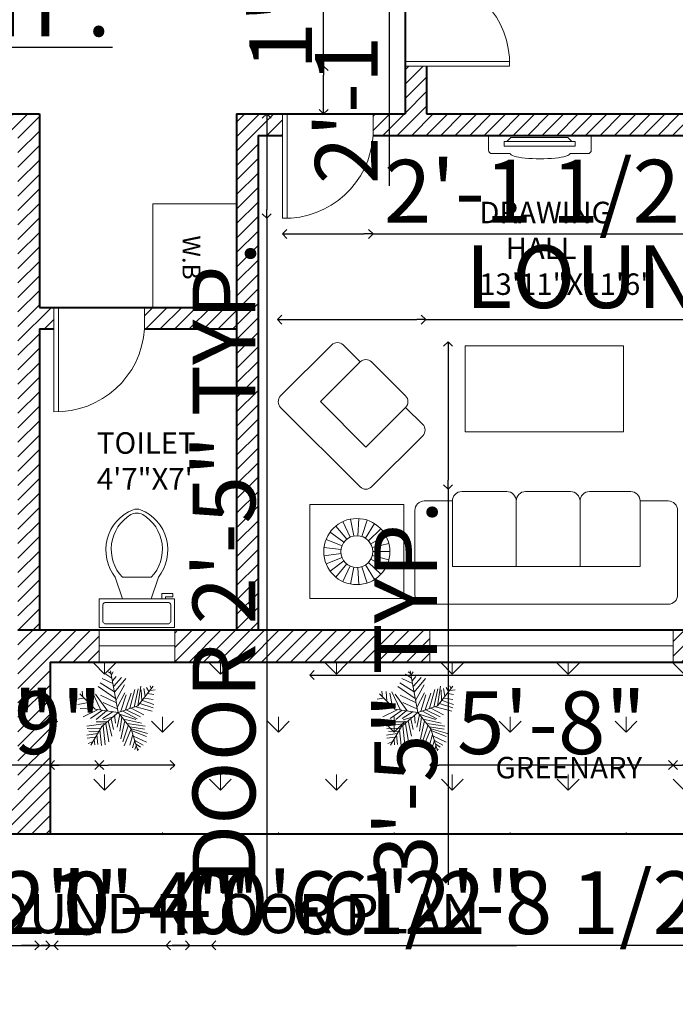
# Model space of a CAD drawing. Units: inches. Extents: x 597 to 1323, y 1833 to 2686.
# Tile 2 of 10: x 865 to 1048, y 1896 to 2171. Entities that reach past the tile are written whole.
import ezdxf

# ---------------------------------------------------------------- set-up
doc = ezdxf.new("R2010")
doc.units = ezdxf.units.IN
for name, color, linetype, lineweight in [('A-ANNO-DIMS', 2, 'Continuous', 18), ('A-ANNO-TEXT', 7, 'Continuous', 18), ('A-AREA-IDEN', 7, 'Continuous', 18), ('A-DOOR', 5, 'Continuous', 20), ('A-EQPM', 8, 'Continuous', 18), ('A-FLOR-FIXT', 4, 'Continuous', 18), ('A-FURN', 8, 'Continuous', 18), ('A-GLAZ', 2, 'Continuous', 18), ('A-WALL', 7, 'Continuous', 40), ('A-WALL-PATT', 8, 'Continuous', 13), ('L-PLNT', 3, 'Continuous', 18), ('L-PLNT-PATT', 3, 'Continuous', 13), ('SOFA', 10, 'Continuous', 18)]:
    doc.layers.add(name, color=color, linetype=linetype, lineweight=lineweight)
doc.styles.get("Standard").update_dxf_attribs({"font": 'arial.ttf'})
doc.dimstyles.new('ISO-25', dxfattribs={"dimtxt": 17.5, "dimasz": 2.5, "dimexe": 0, "dimexo": 0, "dimtad": 1, "dimdec": 1, "dimlunit": 3, "dimtxsty": 'Standard', "dimblk": 'OPEN90', "dimcen": 2.5, "dimadec": 0, "dimazin": 0, "dimtfac": 1, "dimtdec": 1, "dimtmove": 0, "dimatfit": 3, "dimfxl": 0, "dimfxlon": 1, "dimarcsym": 0})

# ---------------------------------------------------------------- blocks, each defined once
blk = doc.blocks.new('*U2')
for p, q in [((-10.186, 53.64), (-13.084, 55.962)), ((0, 0), (-10.5, 57)), ((-9.099, 51.782), (-6.563, 55.962)), ((-5.114, 28.097), (-24.676, 40.636)), ((-7.288, 39.707), (-21.778, 46.673)), ((-8.737, 47.138), (-17.069, 52.711)), ((-7.65, 43.423), (-2.578, 49.46)), ((-5.839, 35.992), (4.667, 48.067)), ((-5.114, 27.632), (10.463, 46.673)), ((-48.585, 21.131), (-49.309, 29.026)), ((-43.513, 28.561), (-42.427, 15.558)), ((-35.544, 28.097), (-24.314, 3.947)), ((-3.665, 19.273), (-27.574, 35.527)), ((-2.941, 16.486), (8.652, 37.85)), ((16.259, 5.805), (23.142, 31.348)), ((22.055, 7.198), (27.489, 32.277)), ((27, 9), (48, 36)), ((27.127, 9.056), (31.112, 35.992)), ((31.836, 30.883), (32.561, 16.486)), ((35.096, 32.741), (37.27, 22.524)), ((38.719, 34.134), (41.979, 28.561)), ((43.791, 29.954), (51.036, 30.883)), ((44.153, 36.456), (45.239, 32.741)), ((-47.498, 19.737), (-55.83, 18.344)), ((-40.615, 13.7), (-55.105, 10.913)), ((-31.5, 4.5), (-52.5, 25.5)), ((-38.442, 26.239), (-34.819, 7.663)), ((-14.533, 2.09), (-30.834, 25.31)), ((-24.314, 23.917), (-2.941, 13.7)), ((-20.691, 13.7), (-1.129, 4.876)), ((-1.129, 6.734), (9.014, 26.704)), ((3.942, 1.625), (11.187, 24.381)), ((10.101, 3.483), (17.708, 26.239)), ((33.285, 16.486), (48.862, 10.913)), ((36.183, 19.737), (48.137, 17.88)), ((40.53, 25.775), (48.862, 24.846)), ((-33.37, 6.269), (-52.207, 5.34)), ((-28.299, 3.483), (-47.86, -5.805)), ((-21.416, 3.018), (-38.079, -8.128)), ((0, 0), (-31.5, 4.5)), ((-15.982, 2.09), (-30.11, -9.521)), ((0, 0), (-22.5, -19.5)), ((-6.563, 1.161), (-21.416, -8.128)), ((0, 0), (27, 9)), ((0, 0), (18, -22.5)), ((6.478, 1.625), (26.04, -8.592)), ((11.187, 3.483), (30.749, -5.805)), ((18.07, 5.805), (35.096, -3.483)), ((24.229, 7.663), (46.688, 1.625)), ((29.662, 12.307), (48.137, 6.269)), ((-15.257, -12.772), (-30.11, -12.772)), ((-6.563, -5.805), (-19.967, -9.985)), ((-13.446, -11.378), (-8.737, -32.741)), ((-9.461, -8.592), (-6.201, -23.453)), ((-4.752, -3.483), (-3.665, -14.629)), ((2.493, -3.019), (-1.491, -20.202)), ((1.769, -2.555), (24.229, -9.521)), ((5.029, -6.27), (2.131, -25.775)), ((9.014, -11.378), (3.58, -35.992)), ((7.565, -9.056), (32.198, -14.629)), ((-17.431, -15.094), (-42.789, -18.809)), ((-24.314, -21.596), (-42.427, -22.06)), ((-26.849, -26.24), (-40.253, -25.775)), ((-22.5, -19.5), (-37.5, -45)), ((-25.038, -23.918), (-22.865, -45.281)), ((-20.691, -18.345), (-17.793, -44.352)), ((-17.069, -15.094), (-12.721, -40.172)), ((14.085, -16.951), (6.478, -40.172)), ((18.07, -22.524), (8.289, -45.745)), ((12.274, -15.094), (36.907, -18.809)), ((16.259, -19.738), (36.183, -22.989)), ((18, -22.5), (27, -52.5)), ((18.433, -22.524), (40.53, -29.026)), ((19.157, -25.311), (38.719, -33.206)), ((-28.299, -29.026), (-42.789, -31.348)), ((-30.834, -34.135), (-42.427, -35.528)), ((-34.457, -39.708), (-40.978, -42.494)), ((-32.646, -36.921), (-31.921, -44.352)), ((-29.023, -30.884), (-27.936, -43.887)), ((20.244, -30.419), (15.897, -44.816)), ((22.78, -37.85), (19.519, -48.532)), ((21.331, -32.741), (39.081, -40.636)), ((22.78, -38.314), (34.372, -44.816)), ((24.591, -45.745), (23.142, -50.854)), ((24.591, -43.423), (30.749, -47.603)), ((26.764, -49.925), (28.213, -50.854))]:
    blk.add_line(p, q)
blk = doc.blocks.new('*U4')
for p, q in [((9.5, -6), (9.5, -2)), ((-8, -8.5), (-8, -8)), ((-7, -8), (-7, -9.5)), ((-4, -8), (-6, -14)), ((4, -8), (6, -14)), ((-10, -8.5), (-8, -8.5)), ((-10, -9.5), (-10, -8.5)), ((-7, -9.5), (-10, -9.5)), ((4, -14), (-4, -14))]:
    blk.add_line(p, q)
blk.add_lwpolyline([(10.5, -8), (10.5, 0), (-10.5, 0), (-10.5, -8)], close=True)
for points in [[(-9.5, -2), (-9.5, -6)], [(8.5, -1), (-8.5, -1)], [(-8.5, -7), (8.5, -7)]]:
    blk.add_lwpolyline(points)
for centre, radius, start, end in [((-8.62, -1.88), 0.884, 81.8699, 188.1301), ((8.62, -1.88), 0.884, 351.8699, 98.1301), ((-8.62, -6.12), 0.884, 171.8699, 278.1301), ((8.62, -6.12), 0.884, 261.8699, 8.1301), ((3.52, -21.58), 12.17, 141.4691, 247.9714), ((4.2, -21.82), 11.33, 136.3677, 238.9468), ((-3.52, -21.58), 12.17, 292.0284, 38.5307), ((-4.2, -21.82), 11.33, 301.053, 43.6321), ((0, -27.88), 4, 245.7318, 294.2682), ((0, -29), 4, 254.8605, 285.1395)]:
    blk.add_arc(centre, radius, start, end)
blk = doc.blocks.new('new block')
for p, q in [((-74.3, 8.91), (-74.3, 27.23)), ((-56.5, 8.91), (-56.5, 27.23)), ((-119.59, 17.47), (-120.49, 22.18)), ((-118.48, 17.54), (-118.18, 22.32)), ((-13.95, 17.47), (-14.85, 22.18)), ((-12.84, 17.54), (-12.54, 22.32)), ((-121.59, 16.53), (-124.64, 20.23)), ((-120.65, 17.13), (-122.69, 21.46)), ((-117.39, 17.33), (-115.91, 21.89)), ((-116.38, 16.86), (-113.82, 20.91)), ((-115.53, 16.15), (-112.03, 19.43)), ((-15.95, 16.53), (-19, 20.23)), ((-15.01, 17.13), (-17.05, 21.46)), ((-11.75, 17.33), (-10.27, 21.89)), ((-10.74, 16.86), (-8.17, 20.91)), ((-9.89, 16.15), (-6.39, 19.43)), ((-122.88, 14.75), (-127.34, 16.51)), ((-122.35, 15.72), (-126.23, 18.54)), ((-114.87, 15.25), (-110.67, 17.56)), ((-17.24, 14.75), (-21.7, 16.51)), ((-16.71, 15.72), (-20.59, 18.54)), ((-9.23, 15.25), (-5.03, 17.56)), ((-123.16, 13.67), (-127.92, 14.27)), ((-114.47, 14.22), (-109.82, 15.41)), ((-17.52, 13.67), (-22.27, 14.27)), ((-8.82, 14.22), (-4.18, 15.41)), ((-123.16, 12.56), (-127.92, 11.96)), ((-122.88, 11.48), (-127.34, 9.72)), ((-114.47, 12.01), (-109.82, 10.82)), ((-114.33, 13.11), (-109.53, 13.11)), ((-17.52, 12.56), (-22.27, 11.96)), ((-17.24, 11.48), (-21.7, 9.72)), ((-8.82, 12.01), (-4.18, 10.82)), ((-8.68, 13.11), (-3.89, 13.11)), ((-122.35, 10.51), (-126.23, 7.69)), ((-121.59, 9.7), (-124.64, 6)), ((-120.65, 9.1), (-122.69, 4.76)), ((-119.59, 8.76), (-120.49, 4.05)), ((-118.48, 8.69), (-118.18, 3.9)), ((-117.39, 8.9), (-115.91, 4.34)), ((-116.38, 9.37), (-113.82, 5.32)), ((-115.53, 10.08), (-112.03, 6.8)), ((-114.87, 10.98), (-110.67, 8.67)), ((-16.71, 10.51), (-20.59, 7.69)), ((-15.95, 9.7), (-19, 6)), ((-15.01, 9.1), (-17.05, 4.76)), ((-13.95, 8.76), (-14.85, 4.05)), ((-12.84, 8.69), (-12.54, 3.9)), ((-11.75, 8.9), (-10.27, 4.34)), ((-10.74, 9.37), (-8.17, 5.32)), ((-9.89, 10.08), (-6.39, 6.8)), ((-9.23, 10.98), (-5.03, 8.67))]:
    blk.add_line(p, q)
blk.add_lwpolyline([(-56.5, 27.23, 0.414214), (-59.12, 29.85), (-71.69, 29.85, 0.414214), (-74.3, 27.23, 0.414214), (-76.92, 29.85), (-89.49, 29.85, 0.414214), (-92.11, 27.23), (-92.11, 8.91), (-39.75, 8.91), (-39.75, 27.23, 0.414214), (-42.36, 29.85), (-53.88, 29.85, 0.414214)], format="xyb", close=True)
for points in [[(-131.88, 26.23), (-105.64, 26.23), (-105.64, 0), (-131.88, 0)], [(-26.24, 26.23), (0, 26.23), (0, 0), (-26.24, 0)]]:
    blk.add_lwpolyline(points, close=True)
blk.add_lwpolyline([(-92.11, 27.23), (-99.96, 27.23, 0.414214), (-102.58, 24.61), (-102.58, 1.05, 0.414214), (-99.96, -1.57), (-31.89, -1.57, 0.414214), (-29.27, 1.05), (-29.27, 24.61, 0.414214), (-31.89, 27.23), (-39.75, 27.23)], format="xyb")
for centre, radius in [((-118.76, 13.11), 9.23), ((-13.12, 13.11), 9.23), ((-118.76, 13.11), 4.43), ((-13.12, 13.11), 4.43)]:
    blk.add_circle(centre, radius)
blk = doc.blocks.new('DOOR-LEAF-AND-JAMB')
for p, q in [((6, 25.29), (0, 25.29)), ((29.15, 1.29), (0, 1.29)), ((0, 0), (29.15, 0))]:
    blk.add_line(p, q)
blk = doc.blocks.new('LOUNGE-CHAIR')
blk.add_lwpolyline([(18.09, 35.52), (22.84, 40.28, -0.414214), (26.01, 40.28), (40.28, 26.01, -0.414214), (40.28, 22.84), (18.09, 0.66, -0.414214), (14.92, 0.66), (0.66, 14.92, -0.414214), (0.66, 18.09), (5.41, 22.84)], format="xyb")
blk.add_lwpolyline([(5.41, 26.01), (14.92, 35.52, -0.414214), (18.09, 35.52), (29.18, 24.43), (16.5, 11.75), (5.41, 22.84, -0.414214)], format="xyb", close=True)
blk = doc.blocks.new('_Open90')
at = {"color": 0, "linetype": 'ByBlock', "lineweight": -2}
for p, q in [((0, 0), (-1, 0)), ((-0.5, 0.5), (0, 0)), ((0, 0), (-0.5, -0.5))]:
    blk.add_line(p, q, dxfattribs=at)
blk = doc.blocks.new('*D36')
at = {"layer": 'A-ANNO-DIMS', "color": 0, "lineweight": -2, "transparency": 16777216}
for p, q in [((774.39, 2163.19), (778.39, 2163.19)), ((780.89, 2163.19), (891.31, 2163.19))]:
    blk.add_line(p, q, dxfattribs=at)
at = {"layer": 'Defpoints', "color": 0, "transparency": 16777216}
for p in [(771.89, 2173.99), (780.89, 2173.99), (780.89, 2163.19)]:
    blk.add_point(p, dxfattribs=at)
at = {"layer": 'A-ANNO-DIMS', "color": 0, "lineweight": -2, "transparency": 16777216, "xscale": 2.5, "yscale": 2.5, "zscale": 2.5, "rotation": 180}
blk.add_blockref('_Open90', (771.89, 2163.19), dxfattribs=at)
at = {"layer": 'A-ANNO-DIMS', "color": 0, "lineweight": -2, "transparency": 16777216, "xscale": 2.5, "yscale": 2.5, "zscale": 2.5}
blk.add_blockref('_Open90', (780.89, 2163.19), dxfattribs=at)
at = {"layer": 'A-ANNO-DIMS', "color": 0, "transparency": 16777216, "insert": (837.35, 2172.75), "char_height": 17.5, "attachment_point": 5}
blk.add_mtext('0\'-9" TYP.', dxfattribs=at)
blk = doc.blocks.new('*D38')
at = {"layer": 'A-ANNO-DIMS', "color": 0, "lineweight": -2, "transparency": 16777216}
for p, q in [((968.46, 2298.79), (968.46, 2278.5)), ((968.46, 2276), (968.46, 2124.5))]:
    blk.add_line(p, q, dxfattribs=at)
at = {"layer": 'Defpoints', "color": 0, "transparency": 16777216}
for p in [(972.89, 2301.29), (968.46, 2276), (972.89, 2276)]:
    blk.add_point(p, dxfattribs=at)
at = {"layer": 'A-ANNO-DIMS', "color": 0, "lineweight": -2, "transparency": 16777216, "xscale": 2.5, "yscale": 2.5, "zscale": 2.5}
for p, rotation in [((968.46, 2301.29), 90), ((968.46, 2276), 270)]:
    blk.add_blockref('_Open90', p, dxfattribs=dict(at, rotation=rotation))
at = {"layer": 'A-ANNO-DIMS', "color": 0, "transparency": 16777216, "insert": (958.79, 2199), "char_height": 17.5, "attachment_point": 5, "rotation": 90}
blk.add_mtext('2\'-1 1/2" TYP.', dxfattribs=at)
blk = doc.blocks.new('*D39')
at = {"layer": 'A-ANNO-DIMS', "color": 0, "lineweight": -2, "transparency": 16777216}
for p, q in [((934.31, 2142.11), (934.31, 2117.96)), ((934.31, 2115.46), (934.31, 1925.77))]:
    blk.add_line(p, q, dxfattribs=at)
at = {"layer": 'Defpoints', "color": 0, "transparency": 16777216}
for p in [(938.68, 2144.61), (934.31, 2115.46), (938.68, 2115.46)]:
    blk.add_point(p, dxfattribs=at)
at = {"layer": 'A-ANNO-DIMS', "color": 0, "lineweight": -2, "transparency": 16777216, "xscale": 2.5, "yscale": 2.5, "zscale": 2.5}
for p, rotation in [((934.31, 2144.61), 90), ((934.31, 2115.46), 270)]:
    blk.add_blockref('_Open90', p, dxfattribs=dict(at, rotation=rotation))
at = {"layer": 'A-ANNO-DIMS', "color": 0, "transparency": 16777216, "insert": (924.63, 2019.36), "char_height": 17.5, "attachment_point": 5, "rotation": 90}
blk.add_mtext('DOOR 2\'-5" TYP.', dxfattribs=at)
blk = doc.blocks.new('*D40')
at = {"layer": 'A-ANNO-DIMS', "color": 0, "lineweight": -2, "transparency": 16777216}
for p, q in [((941.18, 2111.08), (961.47, 2111.08)), ((963.97, 2111.08), (1115.46, 2111.08))]:
    blk.add_line(p, q, dxfattribs=at)
at = {"layer": 'Defpoints', "color": 0, "transparency": 16777216}
for p in [(938.68, 2115.46), (963.97, 2115.46), (963.97, 2111.08)]:
    blk.add_point(p, dxfattribs=at)
at = {"layer": 'A-ANNO-DIMS', "color": 0, "lineweight": -2, "transparency": 16777216, "xscale": 2.5, "yscale": 2.5, "zscale": 2.5, "rotation": 180}
blk.add_blockref('_Open90', (938.68, 2111.08), dxfattribs=at)
at = {"layer": 'A-ANNO-DIMS', "color": 0, "lineweight": -2, "transparency": 16777216, "xscale": 2.5, "yscale": 2.5, "zscale": 2.5}
blk.add_blockref('_Open90', (963.97, 2111.08), dxfattribs=at)
at = {"layer": 'A-ANNO-DIMS', "color": 0, "transparency": 16777216, "insert": (1040.96, 2120.76), "char_height": 17.5, "attachment_point": 5}
blk.add_mtext('2\'-1 1/2" TYP.', dxfattribs=at)
blk = doc.blocks.new('*D43')
at = {"layer": 'A-ANNO-DIMS', "color": 0, "lineweight": -2, "transparency": 16777216}
for p, q in [((939.8, 2087.21), (976.17, 2087.21)), ((978.67, 2087.21), (1321.98, 2087.21))]:
    blk.add_line(p, q, dxfattribs=at)
at = {"layer": 'Defpoints', "color": 0, "transparency": 16777216}
for p in [(978.67, 2087.21), (937.3, 2081.01), (978.67, 2081.01)]:
    blk.add_point(p, dxfattribs=at)
at = {"layer": 'A-ANNO-DIMS', "color": 0, "lineweight": -2, "transparency": 16777216, "xscale": 2.5, "yscale": 2.5, "zscale": 2.5, "rotation": 180}
blk.add_blockref('_Open90', (937.3, 2087.21), dxfattribs=at)
at = {"layer": 'A-ANNO-DIMS', "color": 0, "lineweight": -2, "transparency": 16777216, "xscale": 2.5, "yscale": 2.5, "zscale": 2.5}
blk.add_blockref('_Open90', (978.67, 2087.21), dxfattribs=at)
at = {"layer": 'A-ANNO-DIMS', "color": 0, "transparency": 16777216, "insert": (1151.58, 2096.9), "char_height": 17.5, "attachment_point": 5}
blk.add_mtext('LOUNGE CHAIR 3\'-5 1/2" TYP.', dxfattribs=at)
blk = doc.blocks.new('*D44')
at = {"layer": 'A-ANNO-DIMS', "color": 0, "lineweight": -2, "transparency": 16777216}
for p, q in [((984.87, 2078.51), (984.87, 2042.35)), ((984.87, 2039.85), (984.87, 1929.44))]:
    blk.add_line(p, q, dxfattribs=at)
at = {"layer": 'Defpoints', "color": 0, "transparency": 16777216}
for p in [(978.67, 2081.01), (978.67, 2039.85), (984.87, 2039.85)]:
    blk.add_point(p, dxfattribs=at)
at = {"layer": 'A-ANNO-DIMS', "color": 0, "lineweight": -2, "transparency": 16777216, "xscale": 2.5, "yscale": 2.5, "zscale": 2.5}
for p, rotation in [((984.87, 2081.01), 90), ((984.87, 2039.85), 270)]:
    blk.add_blockref('_Open90', p, dxfattribs=dict(at, rotation=rotation))
at = {"layer": 'A-ANNO-DIMS', "color": 0, "transparency": 16777216, "insert": (975.31, 1983.4), "char_height": 17.5, "attachment_point": 5, "rotation": 90}
blk.add_mtext('3\'-5" TYP.', dxfattribs=at)
blk = doc.blocks.new('*D51')
at = {"layer": 'A-ANNO-DIMS', "color": 0, "lineweight": -2, "transparency": 16777216}
for p, q in [((948.81, 1987.99), (1075.69, 1987.99)), ((1078.19, 1987.99), (1311.77, 1987.99))]:
    blk.add_line(p, q, dxfattribs=at)
at = {"layer": 'Defpoints', "color": 0, "transparency": 16777216}
for p in [(946.31, 2007.77), (1078.19, 2007.77), (1078.19, 1987.99)]:
    blk.add_point(p, dxfattribs=at)
at = {"layer": 'A-ANNO-DIMS', "color": 0, "lineweight": -2, "transparency": 16777216, "xscale": 2.5, "yscale": 2.5, "zscale": 2.5, "rotation": 180}
blk.add_blockref('_Open90', (946.31, 1987.99), dxfattribs=at)
at = {"layer": 'A-ANNO-DIMS', "color": 0, "lineweight": -2, "transparency": 16777216, "xscale": 2.5, "yscale": 2.5, "zscale": 2.5}
blk.add_blockref('_Open90', (1078.19, 1987.99), dxfattribs=at)
at = {"layer": 'A-ANNO-DIMS', "color": 0, "transparency": 16777216, "insert": (1196.23, 1997.67), "char_height": 17.5, "attachment_point": 5}
blk.add_mtext('SOFA GROUP 11\'-0"', dxfattribs=at)
blk = doc.blocks.new('*D55')
at = {"layer": 'A-ANNO-DIMS', "color": 0, "lineweight": -2, "transparency": 16777216}
for p, q in [((825.39, 2452.36), (862.39, 2452.36)), ((864.89, 2452.36), (915.14, 2452.36))]:
    blk.add_line(p, q, dxfattribs=at)
at = {"layer": 'Defpoints', "color": 0, "transparency": 16777216}
for p in [(864.89, 2452.36), (822.89, 2075.33), (864.89, 2075.33)]:
    blk.add_point(p, dxfattribs=at)
at = {"layer": 'A-ANNO-DIMS', "color": 0, "lineweight": -2, "transparency": 16777216, "xscale": 2.5, "yscale": 2.5, "zscale": 2.5, "rotation": 180}
blk.add_blockref('_Open90', (822.89, 2452.36), dxfattribs=at)
at = {"layer": 'A-ANNO-DIMS', "color": 0, "lineweight": -2, "transparency": 16777216, "xscale": 2.5, "yscale": 2.5, "zscale": 2.5}
blk.add_blockref('_Open90', (864.89, 2452.36), dxfattribs=at)
at = {"layer": 'A-ANNO-DIMS', "color": 0, "transparency": 16777216, "insert": (891.27, 2461.93), "char_height": 17.5, "attachment_point": 5}
blk.add_mtext('3\'-6"', dxfattribs=at)
blk = doc.blocks.new('*D58')
at = {"layer": 'A-ANNO-DIMS', "color": 0, "lineweight": -2, "transparency": 16777216}
for p, q in [((783.39, 1912.53), (787.76, 1912.53)), ((790.26, 1912.53), (881.3, 1912.53))]:
    blk.add_line(p, q, dxfattribs=at)
at = {"layer": 'Defpoints', "color": 0, "transparency": 16777216}
for p in [(780.89, 1952.61), (790.26, 1952.61), (790.26, 1912.53)]:
    blk.add_point(p, dxfattribs=at)
at = {"layer": 'A-ANNO-DIMS', "color": 0, "lineweight": -2, "transparency": 16777216, "xscale": 2.5, "yscale": 2.5, "zscale": 2.5, "rotation": 180}
blk.add_blockref('_Open90', (780.89, 1912.53), dxfattribs=at)
at = {"layer": 'A-ANNO-DIMS', "color": 0, "lineweight": -2, "transparency": 16777216, "xscale": 2.5, "yscale": 2.5, "zscale": 2.5}
blk.add_blockref('_Open90', (790.26, 1912.53), dxfattribs=at)
at = {"layer": 'A-ANNO-DIMS', "color": 0, "transparency": 16777216, "insert": (837.03, 1922.21), "char_height": 17.5, "attachment_point": 5}
blk.add_mtext('0\'-9 1/2"', dxfattribs=at)
blk = doc.blocks.new('*D59')
at = {"layer": 'A-ANNO-DIMS', "color": 0, "lineweight": -2, "transparency": 16777216}
for p, q in [((910.39, 1912.53), (907.89, 1912.53)), ((912.89, 1912.53), (918.89, 1912.53)), ((921.39, 1912.53), (971.66, 1912.53))]:
    blk.add_line(p, q, dxfattribs=at)
at = {"layer": 'Defpoints', "color": 0, "transparency": 16777216}
for p in [(912.89, 2270.61), (918.89, 2264.61), (918.89, 1912.53)]:
    blk.add_point(p, dxfattribs=at)
at = {"layer": 'A-ANNO-DIMS', "color": 0, "lineweight": -2, "transparency": 16777216, "xscale": 2.5, "yscale": 2.5, "zscale": 2.5}
blk.add_blockref('_Open90', (912.89, 1912.53), dxfattribs=at)
at = {"layer": 'A-ANNO-DIMS', "color": 0, "lineweight": -2, "transparency": 16777216, "xscale": 2.5, "yscale": 2.5, "zscale": 2.5, "rotation": 180}
blk.add_blockref('_Open90', (918.89, 1912.53), dxfattribs=at)
at = {"layer": 'A-ANNO-DIMS', "color": 0, "transparency": 16777216, "insert": (947.77, 1922.09), "char_height": 17.5, "attachment_point": 5}
blk.add_mtext('0\'-6"', dxfattribs=at)
blk = doc.blocks.new('*D67')
at = {"layer": 'A-ANNO-DIMS', "color": 0, "lineweight": -2, "transparency": 16777216}
blk.add_line((1045.15, 1962.86), (982.31, 1962.86), dxfattribs=at)
at = {"layer": 'Defpoints', "color": 0, "transparency": 16777216}
for p in [(979.81, 1991.61), (1047.65, 1991.61), (979.81, 1962.86)]:
    blk.add_point(p, dxfattribs=at)
at = {"layer": 'A-ANNO-DIMS', "color": 0, "lineweight": -2, "transparency": 16777216, "xscale": 2.5, "yscale": 2.5, "zscale": 2.5, "rotation": 180}
blk.add_blockref('_Open90', (979.81, 1962.86), dxfattribs=at)
at = {"layer": 'A-ANNO-DIMS', "color": 0, "lineweight": -2, "transparency": 16777216, "xscale": 2.5, "yscale": 2.5, "zscale": 2.5}
blk.add_blockref('_Open90', (1047.65, 1962.86), dxfattribs=at)
at = {"layer": 'A-ANNO-DIMS', "color": 0, "transparency": 16777216, "insert": (1013.73, 1972.42), "char_height": 17.5, "attachment_point": 5}
blk.add_mtext('5\'-8"', dxfattribs=at)
blk = doc.blocks.new('*D68')
at = {"layer": 'A-ANNO-DIMS', "color": 0, "lineweight": -2, "transparency": 16777216}
for p, q in [((887.56, 1962.86), (838.94, 1962.86)), ((906.12, 1962.86), (890.06, 1962.86))]:
    blk.add_line(p, q, dxfattribs=at)
at = {"layer": 'Defpoints', "color": 0, "transparency": 16777216}
for p in [(887.56, 1991.61), (908.62, 1991.61), (887.56, 1962.86)]:
    blk.add_point(p, dxfattribs=at)
at = {"layer": 'A-ANNO-DIMS', "color": 0, "lineweight": -2, "transparency": 16777216, "xscale": 2.5, "yscale": 2.5, "zscale": 2.5, "rotation": 180}
blk.add_blockref('_Open90', (887.56, 1962.86), dxfattribs=at)
at = {"layer": 'A-ANNO-DIMS', "color": 0, "lineweight": -2, "transparency": 16777216, "xscale": 2.5, "yscale": 2.5, "zscale": 2.5}
blk.add_blockref('_Open90', (908.62, 1962.86), dxfattribs=at)
at = {"layer": 'A-ANNO-DIMS', "color": 0, "transparency": 16777216, "insert": (862, 1972.42), "char_height": 17.5, "attachment_point": 5}
blk.add_mtext('1\'-9"', dxfattribs=at)
blk = doc.blocks.new('*D70')
at = {"layer": 'A-ANNO-DIMS', "color": 0, "lineweight": -2, "transparency": 16777216}
for p, q in [((1066.43, 1912.53), (975.08, 1912.53)), ((1096.39, 1912.53), (1068.93, 1912.53))]:
    blk.add_line(p, q, dxfattribs=at)
at = {"layer": 'Defpoints', "color": 0, "transparency": 16777216}
for p in [(1066.43, 2310.73), (1098.89, 2310.73), (1066.43, 1912.53)]:
    blk.add_point(p, dxfattribs=at)
at = {"layer": 'A-ANNO-DIMS', "color": 0, "lineweight": -2, "transparency": 16777216, "xscale": 2.5, "yscale": 2.5, "zscale": 2.5, "rotation": 180}
blk.add_blockref('_Open90', (1066.43, 1912.53), dxfattribs=at)
at = {"layer": 'A-ANNO-DIMS', "color": 0, "lineweight": -2, "transparency": 16777216, "xscale": 2.5, "yscale": 2.5, "zscale": 2.5}
blk.add_blockref('_Open90', (1098.89, 1912.53), dxfattribs=at)
at = {"layer": 'A-ANNO-DIMS', "color": 0, "transparency": 16777216, "insert": (1019.5, 1922.21), "char_height": 17.5, "attachment_point": 5}
blk.add_mtext('2\'-8 1/2"', dxfattribs=at)
blk = doc.blocks.new('*D76')
at = {"layer": 'A-ANNO-DIMS', "color": 0, "lineweight": -2, "transparency": 16777216}
blk.add_line((1105.39, 1962.86), (1050.15, 1962.86), dxfattribs=at)
at = {"layer": 'Defpoints', "color": 0, "transparency": 16777216}
for p in [(1047.65, 1991.61), (1107.89, 1991.61), (1047.65, 1962.86)]:
    blk.add_point(p, dxfattribs=at)
at = {"layer": 'A-ANNO-DIMS', "color": 0, "lineweight": -2, "transparency": 16777216, "xscale": 2.5, "yscale": 2.5, "zscale": 2.5, "rotation": 180}
blk.add_blockref('_Open90', (1047.65, 1962.86), dxfattribs=at)
at = {"layer": 'A-ANNO-DIMS', "color": 0, "lineweight": -2, "transparency": 16777216, "xscale": 2.5, "yscale": 2.5, "zscale": 2.5}
blk.add_blockref('_Open90', (1107.89, 1962.86), dxfattribs=at)
at = {"layer": 'A-ANNO-DIMS', "color": 0, "transparency": 16777216, "insert": (1077.77, 1972.42), "char_height": 17.5, "attachment_point": 5}
blk.add_mtext('5\'-0"', dxfattribs=at)
blk = doc.blocks.new('*D77')
at = {"layer": 'A-ANNO-DIMS', "color": 0, "lineweight": -2, "transparency": 16777216}
for p, q in [((873.89, 1962.86), (784.49, 1962.86)), ((885.06, 1962.86), (876.39, 1962.86))]:
    blk.add_line(p, q, dxfattribs=at)
at = {"layer": 'Defpoints', "color": 0, "transparency": 16777216}
for p in [(873.89, 1991.61), (887.56, 1991.61), (873.89, 1962.86)]:
    blk.add_point(p, dxfattribs=at)
at = {"layer": 'A-ANNO-DIMS', "color": 0, "lineweight": -2, "transparency": 16777216, "xscale": 2.5, "yscale": 2.5, "zscale": 2.5, "rotation": 180}
blk.add_blockref('_Open90', (873.89, 1962.86), dxfattribs=at)
at = {"layer": 'A-ANNO-DIMS', "color": 0, "lineweight": -2, "transparency": 16777216, "xscale": 2.5, "yscale": 2.5, "zscale": 2.5}
blk.add_blockref('_Open90', (887.56, 1962.86), dxfattribs=at)
at = {"layer": 'A-ANNO-DIMS', "color": 0, "transparency": 16777216, "insert": (827.94, 1972.53), "char_height": 17.5, "attachment_point": 5}
blk.add_mtext('1\'-1 1/2"', dxfattribs=at)
blk = doc.blocks.new('*D78')
at = {"layer": 'A-ANNO-DIMS', "color": 0, "lineweight": -2, "transparency": 16777216}
for p, q in [((860.31, 1912.53), (871.39, 1912.53)), ((873.89, 1912.53), (922.51, 1912.53))]:
    blk.add_line(p, q, dxfattribs=at)
at = {"layer": 'Defpoints', "color": 0, "transparency": 16777216}
for p in [(857.81, 1943.61), (873.89, 1943.61), (873.89, 1912.53)]:
    blk.add_point(p, dxfattribs=at)
at = {"layer": 'A-ANNO-DIMS', "color": 0, "lineweight": -2, "transparency": 16777216, "xscale": 2.5, "yscale": 2.5, "zscale": 2.5, "rotation": 180}
blk.add_blockref('_Open90', (857.81, 1912.53), dxfattribs=at)
at = {"layer": 'A-ANNO-DIMS', "color": 0, "lineweight": -2, "transparency": 16777216, "xscale": 2.5, "yscale": 2.5, "zscale": 2.5}
blk.add_blockref('_Open90', (873.89, 1912.53), dxfattribs=at)
at = {"layer": 'A-ANNO-DIMS', "color": 0, "transparency": 16777216, "insert": (899.45, 1921.95), "char_height": 17.5, "attachment_point": 5}
blk.add_mtext('1\'-4"', dxfattribs=at)
blk = doc.blocks.new('*D79')
at = {"layer": 'A-ANNO-DIMS', "color": 0, "lineweight": -2, "transparency": 16777216}
for p, q in [((908.7, 1912.53), (910.39, 1912.53)), ((912.89, 1912.53), (1003.93, 1912.53))]:
    blk.add_line(p, q, dxfattribs=at)
at = {"layer": 'Defpoints', "color": 0, "transparency": 16777216}
for p in [(906.2, 2270.61), (912.89, 2270.61), (912.89, 1912.53)]:
    blk.add_point(p, dxfattribs=at)
at = {"layer": 'A-ANNO-DIMS', "color": 0, "lineweight": -2, "transparency": 16777216, "xscale": 2.5, "yscale": 2.5, "zscale": 2.5, "rotation": 180}
blk.add_blockref('_Open90', (906.2, 1912.53), dxfattribs=at)
at = {"layer": 'A-ANNO-DIMS', "color": 0, "lineweight": -2, "transparency": 16777216, "xscale": 2.5, "yscale": 2.5, "zscale": 2.5}
blk.add_blockref('_Open90', (912.89, 1912.53), dxfattribs=at)
at = {"layer": 'A-ANNO-DIMS', "color": 0, "transparency": 16777216, "insert": (959.66, 1922.21), "char_height": 17.5, "attachment_point": 5}
blk.add_mtext('0\'-6 1/2"', dxfattribs=at)
blk = doc.blocks.new('*D81')
at = {"layer": 'A-ANNO-DIMS', "color": 0, "lineweight": -2, "transparency": 16777216}
for p, q in [((950.14, 2157.94), (950.14, 2247.34)), ((950.14, 2147.11), (950.14, 2155.44))]:
    blk.add_line(p, q, dxfattribs=at)
at = {"layer": 'Defpoints', "color": 0, "transparency": 16777216}
for p in [(950.14, 2157.94), (978.89, 2157.94), (978.89, 2144.61)]:
    blk.add_point(p, dxfattribs=at)
at = {"layer": 'A-ANNO-DIMS', "color": 0, "lineweight": -2, "transparency": 16777216, "xscale": 2.5, "yscale": 2.5, "zscale": 2.5}
for p, rotation in [((950.14, 2157.94), 90), ((950.14, 2144.61), 270)]:
    blk.add_blockref('_Open90', p, dxfattribs=dict(at, rotation=rotation))
at = {"layer": 'A-ANNO-DIMS', "color": 0, "transparency": 16777216, "insert": (940.46, 2203.89), "char_height": 17.5, "attachment_point": 5, "rotation": 90}
blk.add_mtext('1\'-1 1/2"', dxfattribs=at)
blk = doc.blocks.new('*D82')
at = {"layer": 'A-ANNO-DIMS', "color": 0, "lineweight": -2, "transparency": 16777216}
for p, q in [((934.39, 2452.36), (936.18, 2452.36)), ((938.68, 2452.36), (988.95, 2452.36))]:
    blk.add_line(p, q, dxfattribs=at)
at = {"layer": 'Defpoints', "color": 0, "transparency": 16777216}
for p in [(938.68, 2452.36), (931.89, 2138.61), (938.68, 2138.61)]:
    blk.add_point(p, dxfattribs=at)
at = {"layer": 'A-ANNO-DIMS', "color": 0, "lineweight": -2, "transparency": 16777216, "xscale": 2.5, "yscale": 2.5, "zscale": 2.5, "rotation": 180}
blk.add_blockref('_Open90', (931.89, 2452.36), dxfattribs=at)
at = {"layer": 'A-ANNO-DIMS', "color": 0, "lineweight": -2, "transparency": 16777216, "xscale": 2.5, "yscale": 2.5, "zscale": 2.5}
blk.add_blockref('_Open90', (938.68, 2452.36), dxfattribs=at)
at = {"layer": 'A-ANNO-DIMS', "color": 0, "transparency": 16777216, "insert": (965.06, 2461.92), "char_height": 17.5, "attachment_point": 5}
blk.add_mtext('0\'-7"', dxfattribs=at)
blk = doc.blocks.new('*D83')
at = {"layer": 'A-ANNO-DIMS', "color": 0, "lineweight": -2, "transparency": 16777216}
for p, q in [((868.39, 1912.53), (865.89, 1912.53)), ((870.89, 1912.53), (874.89, 1912.53)), ((877.39, 1912.53), (927.66, 1912.53))]:
    blk.add_line(p, q, dxfattribs=at)
at = {"layer": 'Defpoints', "color": 0, "transparency": 16777216}
for p in [(870.89, 2084.61), (874.89, 2084.61), (874.89, 1912.53)]:
    blk.add_point(p, dxfattribs=at)
at = {"layer": 'A-ANNO-DIMS', "color": 0, "lineweight": -2, "transparency": 16777216, "xscale": 2.5, "yscale": 2.5, "zscale": 2.5}
blk.add_blockref('_Open90', (870.89, 1912.53), dxfattribs=at)
at = {"layer": 'A-ANNO-DIMS', "color": 0, "lineweight": -2, "transparency": 16777216, "xscale": 2.5, "yscale": 2.5, "zscale": 2.5, "rotation": 180}
blk.add_blockref('_Open90', (874.89, 1912.53), dxfattribs=at)
at = {"layer": 'A-ANNO-DIMS', "color": 0, "transparency": 16777216, "insert": (903.78, 1922.09), "char_height": 17.5, "attachment_point": 5}
blk.add_mtext('0\'-4"', dxfattribs=at)

msp = doc.modelspace()

# ---------------------------------------------------------------- hatches: boundary and pattern name
at = {"layer": 'A-WALL-PATT'}
h = msp.add_hatch(dxfattribs=at)
h.set_pattern_fill('ANSI31', color=256, scale=0.9)
h.paths.add_polyline_path([(927.93, 2423.61), (771.89, 2423.61), (771.89, 2371.61), (780.89, 2371.61), (780.89, 2414.61), (918.89, 2414.61), (927.93, 2414.61)])
h.paths.add_polyline_path([(1107.89, 2423.61), (1074.89, 2423.61), (1074.89, 2414.61), (1098.89, 2414.61), (1098.89, 2382.26), (1107.89, 2382.26)])
h.paths.add_polyline_path([(1002.89, 2423.61), (963.93, 2423.61), (963.93, 2414.61), (978.89, 2414.61), (1002.89, 2414.61)])
h.paths.add_polyline_path([(918.89, 2414.61), (912.89, 2414.61), (912.89, 2270.61), (906.2, 2270.61), (906.2, 2264.61), (918.89, 2264.61), (918.89, 2318.61), (928.09, 2318.61), (928.09, 2324.61), (918.89, 2324.61)])
h.paths.add_polyline_path([(780.89, 2299.61), (771.89, 2299.61), (771.89, 2245.99), (780.89, 2245.99)])
h.paths.add_polyline_path([(780.89, 2173.99), (771.89, 2173.99), (771.89, 1943.61), (790.26, 1943.61), (790.26, 1952.61), (780.89, 1952.61)])
h.paths.add_polyline_path([(873.89, 1991.61), (887.56, 1991.61), (887.56, 2000.61), (864.89, 2000.61), (864.89, 1952.61), (857.81, 1952.61), (857.81, 1943.61), (873.89, 1943.61)])
h.paths.add_polyline_path([(979.81, 2000.61), (908.62, 2000.61), (908.62, 1991.61), (979.81, 1991.61)])
h.paths.add_polyline_path([(931.89, 2138.61), (938.68, 2138.61), (938.68, 2144.61), (925.89, 2144.61), (925.89, 2000.61), (931.89, 2000.61)])
h.paths.add_polyline_path([(870.89, 2084.61), (874.89, 2084.61), (874.89, 2090.61), (870.89, 2090.61), (870.89, 2144.61), (815.52, 2144.61), (815.52, 2138.61), (864.89, 2138.61), (864.89, 2000.61), (870.89, 2000.61)])
h.paths.add_polyline_path([(925.89, 2090.61), (900.18, 2090.61), (900.18, 2084.61), (925.89, 2084.61)])
h.paths.add_polyline_path([(1107.89, 2051.2), (1098.89, 2051.2), (1098.89, 2000.61), (1047.65, 2000.61), (1047.65, 1991.61), (1107.89, 1991.61)])
h.paths.add_polyline_path([(1107.89, 2181.44), (1098.89, 2181.44), (1098.89, 2109.76), (1107.89, 2109.76)])
h.paths.add_polyline_path([(1098.89, 2144.61), (978.89, 2144.61), (978.89, 2157.94), (972.89, 2157.94), (972.89, 2144.61), (963.97, 2144.61), (963.97, 2138.61), (1098.89, 2138.61)])
h.paths.add_polyline_path([(1107.89, 2310.26), (1098.89, 2310.26), (1098.89, 2227.53), (1107.89, 2227.53)])
h.paths.add_polyline_path([(1098.89, 2270.61), (978.89, 2270.61), (978.89, 2276), (972.89, 2276), (972.89, 2183.23), (978.89, 2183.23), (978.89, 2264.61), (1098.89, 2264.61)])
h.paths.add_polyline_path([(880.92, 2270.61), (780.89, 2270.61), (780.89, 2264.61), (880.92, 2264.61)])
h.paths.add_polyline_path([(978.89, 2414.61), (972.89, 2414.61), (972.89, 2324.61), (961.07, 2324.61), (961.07, 2318.61), (972.89, 2318.61), (972.89, 2301.29), (978.89, 2301.29)])
h.paths.add_polyline_path([(790.26, 2144.61), (780.89, 2144.61), (780.89, 2138.61), (790.26, 2138.61)], flags=17)
at = {"layer": 'L-PLNT-PATT'}
h = msp.add_hatch(dxfattribs=at)
h.set_pattern_fill('GRASS', color=256, scale=0.9)
h.paths.add_polyline_path([(1107.89, 1991.61), (873.89, 1991.61), (873.89, 1943.61), (1107.89, 1943.61)])
h.paths.add_polyline_path([(897.46, 1969.81), (897.45, 1969.79), (897.46, 1969.78)], flags=16)
h.paths.add_polyline_path([(887.13, 1971.67), (886.91, 1971.63), (886.94, 1971.34)], flags=16)
h.paths.add_polyline_path([(891.46, 1976.37), (890.84, 1976.17), (890.9, 1975.88)], flags=16)
h.paths.add_polyline_path([(889.89, 1977.98), (889.78, 1978.14), (889.63, 1978.02)], flags=16)
h.paths.add_polyline_path([(890.92, 1987.98), (891.07, 1988.23), (890.84, 1988.41)], flags=16)
h.paths.add_polyline_path([(896.52, 1973), (896.51, 1972.97), (892.84, 1977.56), (894.89, 1978.24), (894.93, 1978.36), (895.05, 1978.3), (896.12, 1978.66), (896.19, 1978.92), (896.47, 1978.77), (898.33, 1979.39), (899.47, 1980.85), (899.46, 1980.97), (899.54, 1980.94), (898.36, 1979.43), (898.36, 1979.4), (892.84, 1977.56), (893.28, 1977.02), (893.36, 1976.99), (893.35, 1976.93), (894.3, 1975.74), (894.76, 1975.64), (894.68, 1975.27), (895.29, 1974.5), (895.81, 1974.42), (895.67, 1974.02), (896.48, 1973.02)], flags=16)
h.paths.add_polyline_path([(970.73, 1971.67), (970.51, 1971.63), (970.54, 1971.34)], flags=16)
h.paths.add_polyline_path([(973.49, 1977.98), (973.38, 1978.14), (973.23, 1978.02)], flags=16)
h.paths.add_polyline_path([(966.92, 1981.6), (966.59, 1981.54), (966.55, 1981.96), (969.68, 1978.84), (969.42, 1978.83), (969.35, 1979.16)], flags=16)
h.paths.add_polyline_path([(975.06, 1976.37), (974.44, 1976.17), (974.5, 1975.88)], flags=16)
h.paths.add_polyline_path([(974.52, 1987.98), (974.67, 1988.23), (974.44, 1988.41)], flags=16)
h.paths.add_polyline_path([(886.08, 1978.84), (885.82, 1978.83), (885.75, 1979.16), (883.32, 1981.6), (882.99, 1981.54), (882.95, 1981.96)], flags=16)
h.paths.add_polyline_path([(981.05, 1969.81), (981.05, 1969.79), (981.06, 1969.78)], flags=16)
h.paths.add_polyline_path([(976.44, 1977.56), (978.49, 1978.24), (978.52, 1978.36), (978.65, 1978.3), (979.72, 1978.66), (979.79, 1978.92), (980.06, 1978.77), (981.93, 1979.39), (983.06, 1980.85), (983.06, 1980.97), (983.14, 1980.94), (981.96, 1979.43), (981.96, 1979.4), (976.44, 1977.56), (976.87, 1977.02), (976.96, 1976.99), (976.94, 1976.93), (977.9, 1975.74), (978.36, 1975.64), (978.28, 1975.27), (978.89, 1974.5), (979.41, 1974.42), (979.27, 1974.02), (980.08, 1973.02), (980.12, 1973), (980.11, 1972.97)], flags=16)
h.paths.add_polyline_path([(1063.75, 1977.98), (1063.64, 1978.14), (1063.5, 1978.02)], flags=16)
h.paths.add_polyline_path([(1057.18, 1981.6), (1056.86, 1981.54), (1056.82, 1981.96), (1059.94, 1978.84), (1059.68, 1978.83), (1059.62, 1979.16)], flags=16)
h.paths.add_polyline_path([(1065.33, 1976.37), (1064.7, 1976.17), (1064.77, 1975.88)], flags=16)
h.paths.add_polyline_path([(1060.77, 1971.63), (1060.8, 1971.34), (1061, 1971.67)], flags=16)
h.paths.add_polyline_path([(1064.79, 1987.98), (1064.94, 1988.23), (1064.71, 1988.41)], flags=16)
h.paths.add_polyline_path([(1071.32, 1969.81), (1071.31, 1969.79), (1071.33, 1969.78)], flags=16)
h.paths.add_polyline_path([(1066.71, 1977.56), (1068.75, 1978.24), (1068.79, 1978.36), (1068.92, 1978.3), (1069.99, 1978.66), (1070.06, 1978.92), (1070.33, 1978.77), (1072.19, 1979.39), (1073.33, 1980.85), (1073.32, 1980.97), (1073.4, 1980.94), (1072.22, 1979.43), (1072.22, 1979.4), (1066.71, 1977.56), (1067.14, 1977.02), (1067.22, 1976.99), (1067.21, 1976.93), (1068.16, 1975.74), (1068.62, 1975.64), (1068.54, 1975.27), (1069.15, 1974.5), (1069.67, 1974.42), (1069.54, 1974.02), (1070.34, 1973.02), (1070.39, 1973), (1070.38, 1972.97)], flags=16)

# ---------------------------------------------------------------- linework, layer by layer
at = {"layer": 'A-DOOR'}
for centre, radius, start, end in [((977.34, 2158.57), 24.7, 358.539, 86.4204), ((939.32, 2140.14), 24.69, 268.5075, 356.4519), ((939.32, 2140.12), 24.67, 268.5063, 271.4937), ((875.54, 2086.14), 24.68, 268.52, 356.4442)]:
    msp.add_arc(centre, radius, start, end, dxfattribs=at)
at = {"layer": 'A-EQPM'}
for p, q in [((996.17, 2138.61), (996.17, 2134.5)), ((1001.28, 2136.9), (1002.42, 2138.05)), ((1002.42, 2138.05), (1018.26, 2138.05)), ((1018.26, 2138.05), (1019.4, 2136.9)), ((1024.84, 2134.5), (1024.84, 2138.61)), ((997.17, 2133.5), (1002.24, 2133.5)), ((1018.89, 2133.5), (1023.84, 2133.5))]:
    msp.add_line(p, q, dxfattribs=at)
msp.add_lwpolyline([(1000.57, 2136.9), (1020.31, 2136.9), (1020.31, 2135.58), (1000.57, 2135.58)], close=True, dxfattribs=at)
for centre, start, end in [((997.17, 2134.5), 180, 270), ((1023.84, 2134.5), 270, 0)]:
    msp.add_arc(centre, 1, start, end, dxfattribs=at)
msp.add_ellipse((1010.56, 2133.5), major_axis=(-8.33, 0), ratio=0.171474, start_param=0, end_param=3.141593, dxfattribs=at)
at = {"layer": 'A-FLOR-FIXT'}
for p, q in [((902.55, 2090.61), (902.55, 2119.48)), ((902.55, 2119.48), (925.89, 2119.48))]:
    msp.add_line(p, q, dxfattribs=at)
at = {"layer": 'A-FURN'}
msp.add_lwpolyline([(989.61, 2079.9), (1033.78, 2079.9), (1033.78, 2055.88), (989.61, 2055.88)], close=True, dxfattribs=at)
at = {"layer": 'A-GLAZ'}
for p, q in [((887.56, 2000.61), (887.56, 1991.61)), ((908.62, 2000.61), (908.62, 1991.61)), ((979.81, 2000.61), (979.81, 1991.61)), ((1047.65, 2000.61), (1047.65, 1991.61)), ((887.56, 1996.11), (908.62, 1996.11)), ((979.81, 1996.11), (1047.65, 1996.11))]:
    msp.add_line(p, q, dxfattribs=at)
at = {"layer": 'A-WALL'}
for p, q in [((972.89, 2318.61), (972.89, 2144.61)), ((978.89, 2157.94), (978.89, 2144.61)), ((815.52, 2144.61), (870.89, 2144.61)), ((870.89, 2144.61), (870.89, 2090.61)), ((925.89, 2144.61), (972.89, 2144.61)), ((925.89, 2144.61), (925.89, 2000.61)), ((978.89, 2144.61), (1098.89, 2144.61)), ((931.89, 2138.61), (938.68, 2138.61)), ((931.89, 2138.61), (931.89, 2000.61)), ((963.97, 2138.61), (1098.89, 2138.61)), ((870.89, 2090.61), (925.89, 2090.61)), ((870.89, 2084.61), (874.89, 2084.61)), ((870.89, 2084.61), (870.89, 2000.61)), ((900.18, 2084.61), (925.89, 2084.61)), ((864.89, 2000.61), (1098.89, 2000.61)), ((873.89, 1991.61), (1107.89, 1991.61)), ((873.89, 1991.61), (873.89, 1943.61)), ((1107.89, 1943.61), (771.89, 1943.61))]:
    msp.add_line(p, q, dxfattribs=at)

# ---------------------------------------------------------------- block references
at = {"layer": 'A-DOOR'}
msp.add_blockref('DOOR-LEAF-AND-JAMB', (972.89, 2157.94), dxfattribs=at)
for p, rotation in [((938.68, 2144.61), 270.0000000000007), ((874.89, 2090.61), 270.0000000000021)]:
    msp.add_blockref('DOOR-LEAF-AND-JAMB', p, dxfattribs=dict(at, rotation=rotation))
at = {"layer": 'A-FLOR-FIXT', "rotation": 180}
msp.add_blockref('*U4', (898.06, 2001.28), dxfattribs=at)
at = {"layer": 'L-PLNT', "xscale": 0.2033280951175252, "yscale": 0.2033280951175252, "zscale": 0.2033280951175252}
for p in [(892.84, 1977.56), (976.44, 1977.56)]:
    msp.add_blockref('*U2', p, dxfattribs=at)
at = {"layer": 'SOFA', "rotation": 269.9999999999998}
msp.add_blockref('LOUNGE-CHAIR', (937.52, 2080.79), dxfattribs=at)
at = {"layer": 'SOFA'}
msp.add_blockref('new block', (1078.19, 2009.34), dxfattribs=at)

# ---------------------------------------------------------------- texts
at = {"layer": 'A-ANNO-TEXT', "insert": (836.87, 1926.94), "char_height": 11, "attachment_point": 1}
msp.add_mtext_dynamic_manual_height_columns('GROUND RLOOR PLAN', width=624.2346, gutter_width=12.5, heights=[0], dxfattribs=at)
at = {"layer": 'A-AREA-IDEN', "char_height": 6, "attachment_point": 1}
for s, insert in [('DRAWING\\P    HALL\\P13\'11"X11\'6"', (993.58, 2120.08)), ('TOILET\\P4\'7"X7\'', (886.92, 2055.75)), ('GREENARY', (998.1, 1965.16))]:
    msp.add_mtext_dynamic_manual_height_columns(s, width=54.7527, gutter_width=12.5, heights=[0], dxfattribs=dict(at, insert=insert))
at = {"layer": 'A-AREA-IDEN', "insert": (915.81, 2110.69), "char_height": 5, "attachment_point": 1, "rotation": 270}
msp.add_mtext_dynamic_manual_height_columns('W.B', width=10.478, gutter_width=12.5, heights=[0], dxfattribs=at)

# ---------------------------------------------------------------- dimensions: what is measured, and where the dimension line sits
at = {"layer": 'A-ANNO-DIMS'}
for base, p1, p2, picture, middle in [((864.89, 2452.36), (822.89, 2075.33), (864.89, 2075.33), '*D55', (891.27, 2461.93)), ((938.68, 2452.36), (931.89, 2138.61), (938.68, 2138.61), '*D82', (965.06, 2461.92)), ((1066.43, 1912.53), (1098.89, 2310.73), (1066.43, 2310.73), '*D70', (1019.5, 1922.21)), ((912.89, 1912.53), (906.2, 2270.61), (912.89, 2270.61), '*D79', (959.66, 1922.21)), ((918.89, 1912.53), (912.89, 2270.61), (918.89, 2264.61), '*D59', (947.77, 1922.09)), ((874.89, 1912.53), (870.89, 2084.61), (874.89, 2084.61), '*D83', (903.78, 1922.09)), ((790.26, 1912.53), (780.89, 1952.61), (790.26, 1952.61), '*D58', (837.03, 1922.21)), ((873.89, 1912.53), (857.81, 1943.61), (873.89, 1943.61), '*D78', (899.45, 1921.95))]:
    dim = msp.add_linear_dim(base=base, p1=p1, p2=p2, dimstyle='ISO-25', override={"dimdec": 1, "dimlfac": 1, "dimrnd": 0, "dimzin": 1, "dimdsep": 46, "dimlunit": 4, "dimfrac": 2}, dxfattribs=at)
    dim.commit()
    dim.dimension.update_dxf_attribs({"geometry": picture, "text_midpoint": middle})
for base, p1, p2, text, picture, middle in [((968.46, 2276), (972.89, 2301.29), (972.89, 2276), '<> TYP.', '*D38', (958.79, 2199)), ((934.3067, 2115.4566), (938.6798, 2144.6106), (938.6798, 2115.4566), 'DOOR <> TYP.', '*D39', (924.6273, 2019.3644)), ((984.87, 2039.85), (978.67, 2081.01), (978.67, 2039.85), '<> TYP.', '*D44', (975.31, 1983.4))]:
    dim = msp.add_linear_dim(base=base, p1=p1, p2=p2, angle=270, text=text, dimstyle='ISO-25', override={"dimdec": 1, "dimlfac": 1, "dimrnd": 0, "dimzin": 1, "dimdsep": 46, "dimlunit": 4, "dimfrac": 2}, dxfattribs=at)
    dim.commit()
    dim.dimension.update_dxf_attribs({"geometry": picture, "text_midpoint": middle})
for base, p1, p2, angle, picture, middle in [((950.14, 2157.94), (978.89, 2144.61), (978.89, 2157.94), 90, '*D81', (940.46, 2203.89)), ((873.89, 1962.86), (887.56, 1991.61), (873.89, 1991.61), 180, '*D77', (827.94, 1972.53)), ((887.56, 1962.86), (908.62, 1991.61), (887.56, 1991.61), 180, '*D68', (862, 1972.42)), ((979.81, 1962.86), (1047.65, 1991.61), (979.81, 1991.61), 180, '*D67', (1013.73, 1972.42)), ((1047.65, 1962.86), (1107.89, 1991.61), (1047.65, 1991.61), 180, '*D76', (1077.77, 1972.42))]:
    dim = msp.add_linear_dim(base=base, p1=p1, p2=p2, angle=angle, dimstyle='ISO-25', override={"dimdec": 1, "dimlfac": 1, "dimrnd": 0, "dimzin": 1, "dimdsep": 46, "dimlunit": 4, "dimfrac": 2}, dxfattribs=at)
    dim.commit()
    dim.dimension.update_dxf_attribs({"geometry": picture, "text_midpoint": middle})
for base, p1, p2, text, picture, middle in [((780.89, 2163.19), (771.89, 2173.99), (780.89, 2173.99), '<> TYP.', '*D36', (837.35, 2172.75)), ((978.67, 2087.21), (937.3, 2081.01), (978.67, 2081.01), 'LOUNGE CHAIR <> TYP.', '*D43', (1151.58, 2096.9)), ((963.97, 2111.08), (938.68, 2115.46), (963.97, 2115.46), '<> TYP.', '*D40', (1040.96, 2120.76)), ((1078.19, 1987.99), (946.31, 2007.77), (1078.19, 2007.77), 'SOFA GROUP <>', '*D51', (1196.23, 1997.67))]:
    dim = msp.add_linear_dim(base=base, p1=p1, p2=p2, text=text, dimstyle='ISO-25', override={"dimdec": 1, "dimlfac": 1, "dimrnd": 0, "dimzin": 1, "dimdsep": 46, "dimlunit": 4, "dimfrac": 2}, dxfattribs=at)
    dim.commit()
    dim.dimension.update_dxf_attribs({"geometry": picture, "text_midpoint": middle})

doc.saveas('drawing.dxf')
